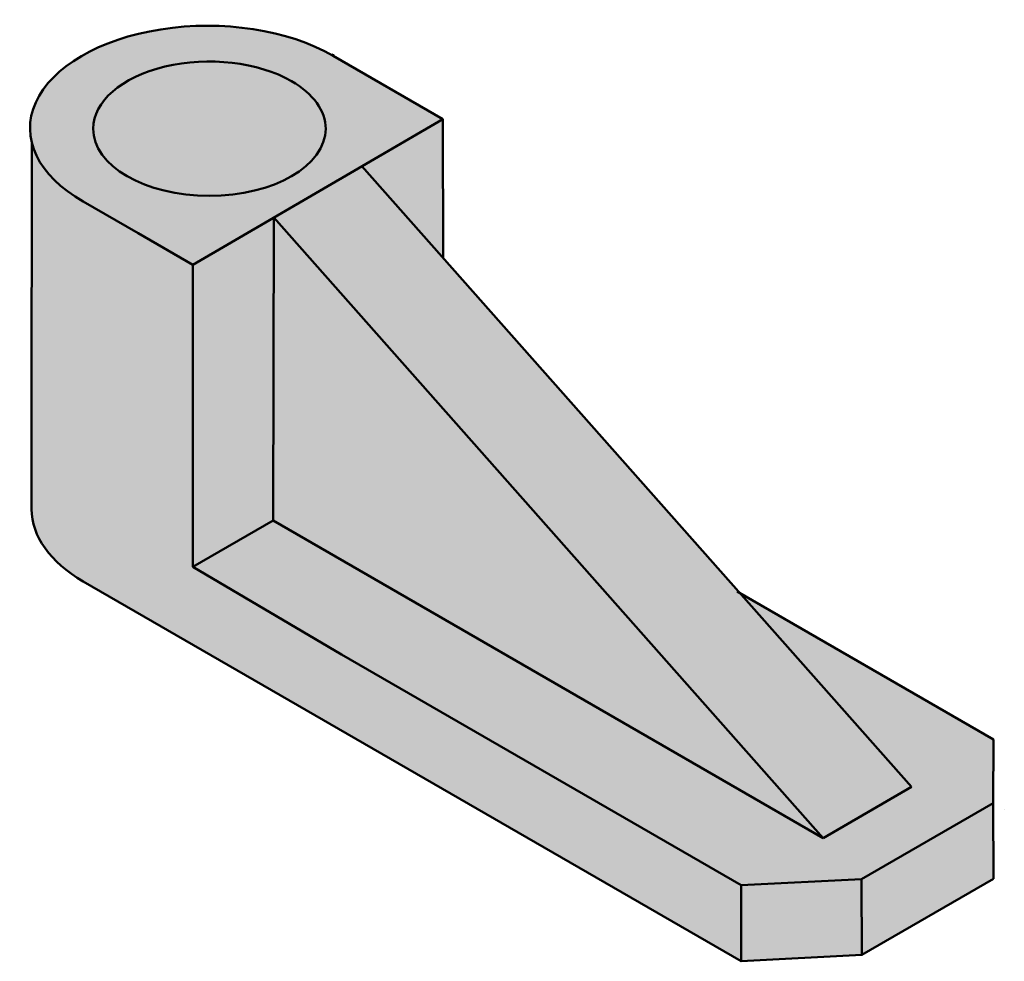
# Model space of a CAD drawing. Units: millimetres. Extents: x 172.3 to 250.1, y 10.1 to 84.5.
import ezdxf

# ---------------------------------------------------------------- set-up
doc = ezdxf.new("R2010")
doc.units = ezdxf.units.MM
doc.header["$MEASUREMENT"] = 0
doc.layers.add('M-HATC', color=252, linetype='Continuous', lineweight=18)
doc.layers.add('M-OUTL', color=7, linetype='Continuous', lineweight=50)

msp = doc.modelspace()

# ---------------------------------------------------------------- hatches: boundary and pattern name
at = {"layer": 'M-HATC'}
h = msp.add_hatch(color=256, dxfattribs=at)
h.dxf.hatch_style = 1
h.paths.add_polyline_path([(205.7128436542433, 76.60700815694601), (199.3197588065982, 72.87689143266913), (205.7442100850354, 65.62763795421574)])
edge = h.paths.add_edge_path()
edge.add_line((205.7128436542433, 76.60700815694601), (197.0525896163989, 81.60700815694594))
edge.add_ellipse((187.1385785768527, 75.88219964634906), major_axis=(-14.02169434630682, 0), ratio=0.5773502691896263, start_angle=210.0041243579652, end_angle=210.5210247195948)
edge.add_ellipse((187.1385785768527, 75.88219964634906), major_axis=(-14.02169434630682, 0), ratio=0.5773502691896263, start_angle=210.5210247195948, end_angle=364.5674946861601)
edge.add_ellipse((187.1385785768527, 75.88219964634906), major_axis=(-14.02169434630682, 0), ratio=0.5773502691896263, start_angle=364.5674946861601, end_angle=390.5210247195948)
edge.add_line((177.327847304709, 70.09838705582152), (181.657974323631, 67.5983870558216))
edge.add_line((181.657974323631, 67.5983870558216), (185.9881013425532, 65.0983870558216))
edge.add_line((185.9881013425532, 65.0983870558216), (205.7128436542433, 76.60700815694601))
h.paths.add_polyline_path([(199.3197588065982, 72.87689143266913), (192.3735638589904, 68.82405644586251), (235.7558584894248, 19.83181504153189), (242.7505750045059, 23.87021650441911)])
h = msp.add_hatch(color=256, dxfattribs=at)
h.dxf.hatch_style = 1
edge = h.paths.add_edge_path()
edge.add_line((185.9881013425532, 65.0983870558216), (181.657974323631, 67.5983870558216))
edge.add_line((181.657974323631, 67.5983870558216), (177.327847304709, 70.0983870558215))
edge.add_ellipse((187.1385785768527, 75.88219964634906), major_axis=(-14.02169434630682, 0), ratio=0.5773502691896263, start_angle=364.56749468616005, end_angle=390.5210247195948, ccw=False)
edge.add_line((173.2492156977313, 74.77261847110947), (173.2461534991674, 51.8534962703818))
edge.add_line((173.2461534991674, 51.8534962703818), (173.2426791078132, 45.79246076931293))
edge.add_ellipse((187.1902107722745, 45.79246076933514), major_axis=(-13.94753166446135, 0), ratio=0.5773502691896258, start_angle=360.0000000000917, end_angle=390.0001547252036)
edge.add_line((177.3278473047088, 40.09838705582161), (229.2893715317751, 10.09838705582164))
edge.add_line((229.2893715317751, 10.09838705582164), (229.2893715317751, 16.09838705582162))
edge.add_line((229.2893715317751, 16.09838705582162), (197.7311907694567, 34.31851121408102))
edge.add_line((197.7311907694567, 34.31851121408102), (185.9835800850913, 41.2393871273839))
edge.add_line((185.9835800850913, 41.2393871273839), (185.9881013425532, 65.0983870558216))
h.paths.add_polyline_path([(192.3735638589904, 68.82405644586251), (192.3252444238055, 44.90649176338791), (206.5828855595025, 36.67483881568419), (235.7558584894248, 19.83181504153186)])
h.paths.add_polyline_path([(206.5828855595025, 36.67483881568419), (192.3252444238055, 44.90649176338791), (185.9835800850913, 41.2393871273839), (197.7311907694568, 34.31851121408089), (229.2893715317751, 16.09838705582162), (238.7926726402509, 16.58512050899021), (249.1965414636594, 22.59179697479862), (249.2223454470745, 27.60669491156949), (229.1888910313747, 39.17301521127188), (242.7505750045059, 23.87021650441912), (235.7558584894248, 19.83181504153187)])
h.paths.add_polyline_path([(192.3735638589904, 68.82405644586252), (185.9881013425532, 65.0983870558216), (185.9835800850913, 41.2393871273839), (192.3252444238055, 44.90649176338791)], flags=17)
h.paths.add_polyline_path([(238.7926726402509, 16.58512050899019), (229.2893715317751, 16.09838705582162), (229.2893715317751, 10.09838705582163), (238.815650973404, 10.59838705582164)])
h.paths.add_polyline_path([(249.2079558188172, 16.59838705582162), (249.1965414636594, 22.59179697479864), (238.7926726402509, 16.58512050899021), (238.815650973404, 10.59838705582166)])
edge = h.paths.add_edge_path()
edge.add_ellipse((186.9282528403045, 75.7582043386177), major_axis=(-9.185586535436917, 0), ratio=0.577350269189626, start_angle=29.999999999999886, end_angle=389.84785620344155, ccw=False)

# ---------------------------------------------------------------- linework, layer by layer
at = {"layer": 'M-OUTL'}
for p, q in [((197.0525896163989, 81.72689972859126), (196.9493098489965, 81.66601223687651)), ((197.0525896163989, 81.60700815694601), (197.0525896163989, 81.72689972859126)), ((197.0525896163989, 81.60700815694601), (205.7128436542433, 76.60700815694601)), ((205.7128436542433, 76.60700815694601), (185.9881013425532, 65.0983870558216)), ((205.7442100850354, 65.62763795421577), (205.7128436542433, 76.60700815694601)), ((173.2461534991674, 51.8534962703818), (173.2492156977313, 74.77261847110948)), ((199.3197588065982, 72.87689143266913), (242.7505750045059, 23.87021650441909)), ((177.3278473047088, 70.0983870558216), (181.657974323631, 67.5983870558216)), ((192.3252444238055, 44.90649176338789), (192.3735638589904, 68.82405644586251)), ((192.3735638589904, 68.82405644586251), (235.7558584894248, 19.83181504153187)), ((181.657974323631, 67.5983870558216), (185.9881013425532, 65.0983870558216)), ((185.9881013425532, 65.0983870558216), (185.9835800850913, 41.2393871273839)), ((173.2426791078132, 45.79246076933514), (173.2461534991674, 51.85349627038199)), ((185.9835800850913, 41.2393871273839), (192.3252444238055, 44.90649176338791)), ((206.5828855595025, 36.67483881568419), (192.3252444238055, 44.9064917633879)), ((185.9835800850913, 41.2393871273839), (197.731190769457, 34.31851121408086)), ((177.3278473047088, 40.09838705582162), (229.2893715317751, 10.09838705582163)), ((249.2223454470745, 27.60669491156949), (228.9625847126376, 39.30367322531404)), ((235.7558584894248, 19.83181504153187), (206.5828855595025, 36.67483881568419)), ((229.2893715317751, 16.09838705582163), (197.731190769457, 34.31851121408086)), ((249.1965414636594, 22.59179697479863), (249.2223454470745, 27.60669491156949)), ((242.7505750045059, 23.87021650441912), (235.7558584894248, 19.83181504153188)), ((249.1965414636594, 22.59179697479863), (238.7926726402509, 16.58512050899021)), ((249.2079558188172, 16.59838705582163), (249.1965414636594, 22.59179697479864)), ((250.0739812226017, 22.09838705582163), (250.0739812226017, 22.09838705582163)), ((229.2893715317751, 16.09838705582163), (238.7926726402509, 16.5851205089902)), ((238.815650973404, 10.59838705582163), (238.7926726402509, 16.5851205089902)), ((238.8156509734039, 10.59838705582162), (249.2079558188172, 16.59838705582164)), ((229.2893715317751, 10.09838705582163), (229.2893715317751, 16.09838705582163)), ((229.2893715317751, 10.09838705582163), (238.815650973404, 10.59838705582163))]:
    msp.add_line(p, q, dxfattribs=at)
for centre, major_axis, ratio, start_param, end_param in [((187.1385785768527, 75.88219964634906), (-14.02169434630682, 0), 0.5773502691896263, 3.927073933064633, 7.079028917192642), ((187.2866538224227, 75.84800000000001), (9.185586535436917, -5e-16), 0.577350269189626, 0.7853981633974482, 3.141592653589793), ((187.2866538224227, 75.84800000000001), (9.185586535436917, -5e-16), 0.577350269189626, 0, 0.7853981633974482), ((187.2866538224227, 75.84800000000001), (9.185586535436917, -5e-16), 0.577350269189626, 3.141592653589793, 6.283185307179586), ((187.1902107722745, 45.79246076933514), (-13.94753166446135, 0), 0.5773502691896258, 6.282523393644032, 7.068586588799683)]:
    msp.add_ellipse(centre, major_axis=major_axis, ratio=ratio, start_param=start_param, end_param=end_param, dxfattribs=at)

doc.saveas('drawing.dxf')
